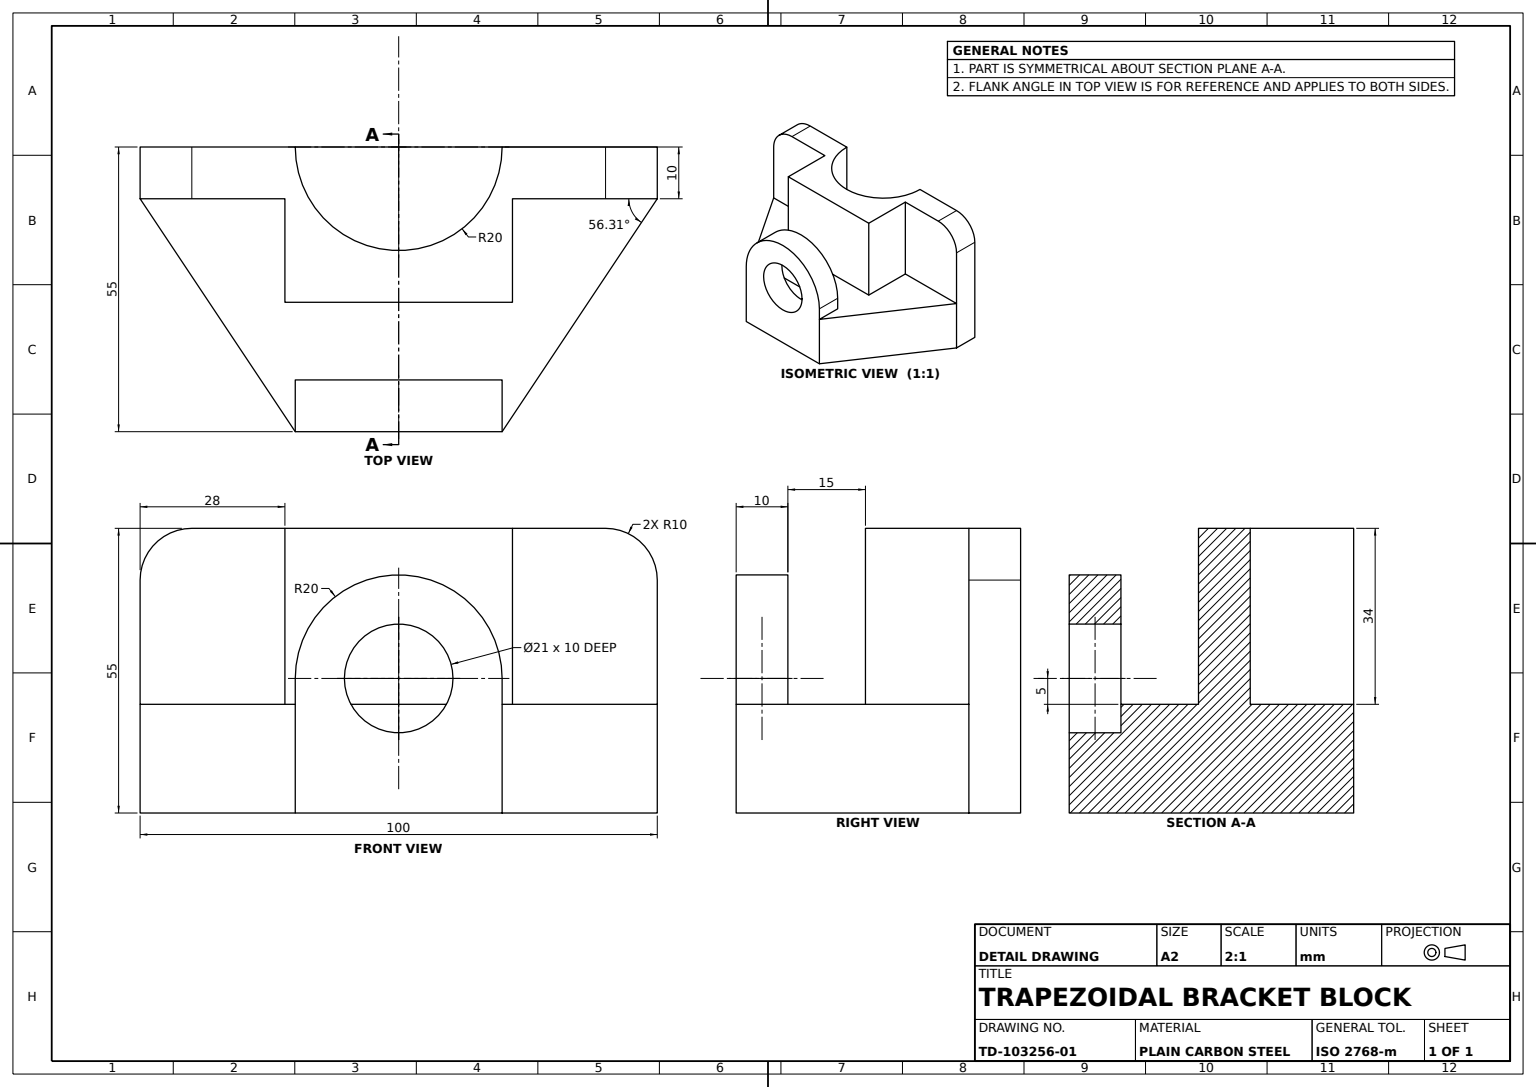
from build123d import *

# Parameters (mm, degrees)
BASE_PROFILE_10MM_DEPTH = 10
UPPER_BLOCK_30MM_DEPTH  = 30
PAD_SKETCH_W            = 44
PAD_SKETCH_H            = 20
PAD_4MM_DEPTH           = 4
PROFILE_CUT_34MM_DEPTH  = 34
SIDE_WALL_21MM_DEPTH    = 21
RAIL_SKETCH_W           = 40
RAIL_SKETCH_H           = 10
RAIL_5MM_DEPTH          = 5
LUG_BOSS_10MM_DEPTH     = 10
LUG_HOLE_SKETCH_21_R    = 10.5
LUG_HOLE_21_DEPTH       = 10


with BuildPart() as part:
    # Base Profile Sketch → Base Profile 10mm (new body)
    with BuildSketch(Plane.XY):
        with BuildLine():
            Line((40, -55), (22, -55))
            Line((22, -55), (22, -25))
            Line((22, -25), (-22, -25))
            Line((-22, -25), (-22, -55))
            Line((-22, -55), (-40, -55))
            ThreePointArc((-40, -55), (-47.071067812, -52.071067812), (-50, -45))
            Line((-50, -45), (-50, 0))
            Line((-50, 0), (0, 0))
            Line((0, 0), (50, 0))
            Line((50, 0), (50, -45))
            ThreePointArc((50, -45), (47.071067812, -52.071067812), (40, -55))
        make_face()
    extrude(amount=BASE_PROFILE_10MM_DEPTH)

    # Upper Block Sketch → Upper Block 30mm (add)
    with BuildSketch(Plane.XZ.offset(25)):
        Polygon((-22, 10), (-22, 30), (22, 30), (22, 10), (22, 0), (-22, 0), align=None)
    extrude(amount=UPPER_BLOCK_30MM_DEPTH)

    # Pad Sketch → Pad 4mm (add)
    with BuildSketch(Plane(origin=(0, -25, 0), x_dir=(1, 0, 0), z_dir=(0, 1, 0))):
        with Locations((0, -20)):
            Rectangle(PAD_SKETCH_W, PAD_SKETCH_H)
    extrude(amount=PAD_4MM_DEPTH)

    # Profile Cut Sketch → Profile Cut 34mm (cut)
    with BuildSketch(Plane.XZ.offset(55)):
        with BuildLine():
            Line((-20, 0), (20, 0))
            ThreePointArc((20, 0), (0, 20), (-20, 0))
        make_face()
    extrude(amount=-PROFILE_CUT_34MM_DEPTH, mode=Mode.SUBTRACT)

    # Side Wall Sketch → Side Wall 21mm (add)
    with BuildSketch(Plane(origin=(0, 0, 0), x_dir=(1, 0, 0), z_dir=(0, 1, 0))):
        Polygon((0, -55), (20, -55), (50, -10), (-50, -10), (-20, -55), align=None)
    extrude(amount=-SIDE_WALL_21MM_DEPTH)

    # Rail Sketch → Rail 5mm (add)
    with BuildSketch(Plane.XZ.offset(21)):
        with Locations((0, 50)):
            Rectangle(RAIL_SKETCH_W, RAIL_SKETCH_H)
    extrude(amount=RAIL_5MM_DEPTH)

    # Lug Sketch → Lug Boss 10mm (add)
    with BuildSketch(Plane.XY.offset(55)):
        with BuildLine():
            Line((-20, -26), (20, -26))
            ThreePointArc((20, -26), (0, -46), (-20, -26))
        make_face()
    extrude(amount=-LUG_BOSS_10MM_DEPTH)

    # Lug Hole Sketch Ø21 → Lug Hole Ø21 (cut)
    with BuildSketch(Plane.XY.offset(55)):
        with Locations((0, -26)):
            Circle(LUG_HOLE_SKETCH_21_R)
    extrude(amount=-LUG_HOLE_21_DEPTH, mode=Mode.SUBTRACT)


solid = part.part
